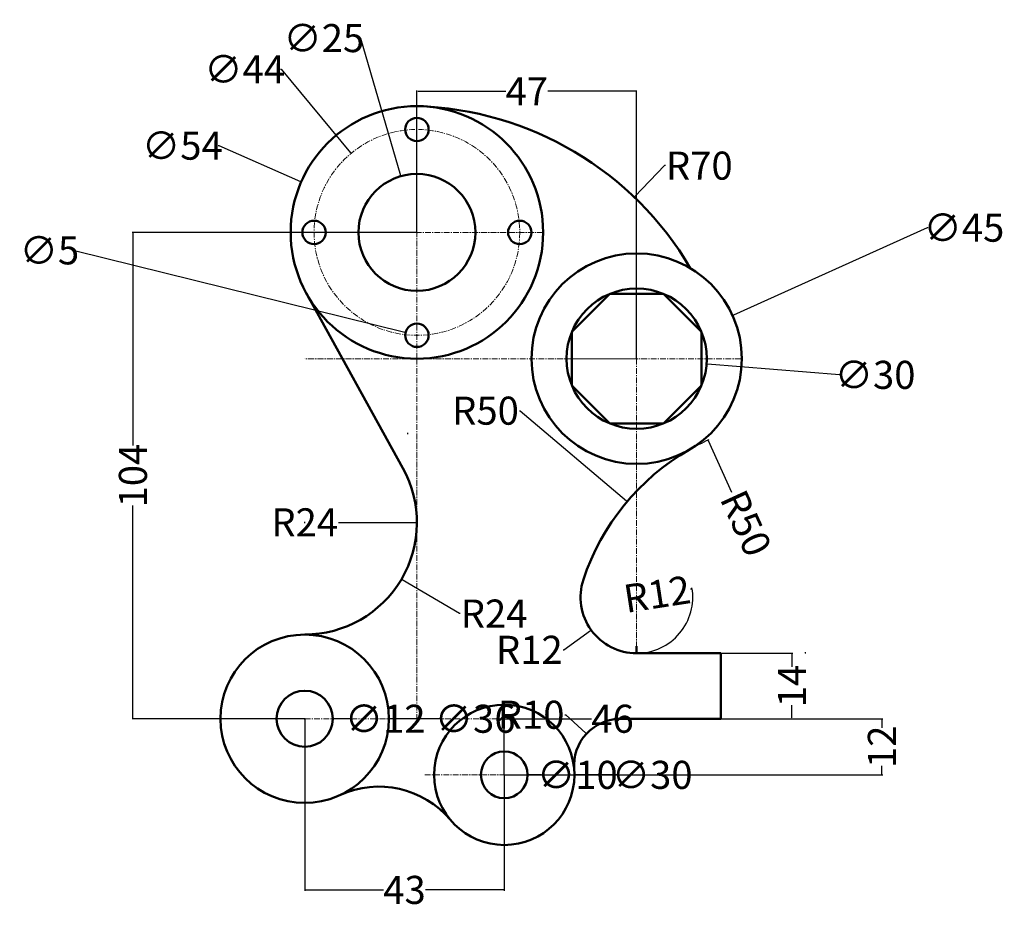
# Model space of a CAD drawing. Units: millimetres. Extents: x 65 to 276, y -19 to 171.
import ezdxf

# ---------------------------------------------------------------- set-up
doc = ezdxf.new("R2010")
doc.units = ezdxf.units.MM
doc.header["$MEASUREMENT"] = 0
doc.linetypes.add('CENTER', pattern=[2, 1.25, -0.25, 0.25, -0.25])
for name, color, linetype, lineweight in [('M-CNTR', 1, 'CENTER', 18), ('M-CONS', 8, 'Continuous', 13), ('M-DIMS', 2, 'Continuous', 25), ('M-OUTL', 7, 'Continuous', 50)]:
    doc.layers.add(name, color=color, linetype=linetype, lineweight=lineweight)
doc.styles.get("Standard").update_dxf_attribs({"font": 'arial.ttf'})
doc.dimstyles.get("Standard").update_dxf_attribs({"dimtxt": 6, "dimasz": 0.18, "dimexe": 0.18, "dimexo": 0.0625, "dimgap": 0.09, "dimtad": 0, "dimtoh": 1, "dimdec": 0, "dimzin": 0, "dimdsep": 46, "dimtxsty": 'Standard', "dimcen": 0.09, "dimadec": 0, "dimazin": 0, "dimtfac": 1, "dimtdec": 0, "dimtofl": 0, "dimtmove": 0, "dimatfit": 3, "dimfxl": 1, "dimtolj": 1, "dimtzin": 0, "dimarcsym": 0})

# ---------------------------------------------------------------- blocks, each defined once
blk = doc.blocks.new('*D1')
at = {"layer": 'Defpoints', "color": 0, "transparency": 16777216}
for p in [(196.83, 132.98), (148.37, 82.46)]:
    blk.add_point(p, dxfattribs=at)
at = {"layer": 'M-DIMS', "color": 0, "lineweight": -2, "transparency": 16777216}
for p, q in [((203.3, 139.72), (196.95, 133.11)), ((203.48, 139.72), (203.3, 139.72)), ((148.28, 82.46), (148.46, 82.46)), ((148.37, 82.37), (148.37, 82.55))]:
    blk.add_line(p, q, dxfattribs=at)
at = {"layer": 'M-DIMS', "color": 0, "transparency": 16777216}
blk.add_solid([(196.93, 133.13), (196.97, 133.09), (196.83, 132.98)], dxfattribs=at)
at = {"layer": 'M-DIMS', "color": 0, "transparency": 16777216, "insert": (210.73, 139.72), "char_height": 6, "attachment_point": 5}
blk.add_mtext('\\A1;R70', dxfattribs=at)
blk = doc.blocks.new('*D2')
at = {"layer": 'Defpoints', "color": 0, "transparency": 16777216}
for p in [(212.6, 81.02), (233.43, 35.56)]:
    blk.add_point(p, dxfattribs=at)
at = {"layer": 'M-DIMS', "color": 0, "lineweight": -2, "transparency": 16777216}
blk.add_line((217.71, 69.85), (212.67, 80.85), dxfattribs=at)
blk.add_arc((233.43, 35.56), 50, 114.4144, 119.7887, dxfattribs=at)
at = {"layer": 'M-DIMS', "color": 0, "transparency": 16777216}
blk.add_solid([(212.7, 80.86), (212.65, 80.84), (212.6, 81.02)], dxfattribs=at)
at = {"layer": 'M-DIMS', "color": 0, "transparency": 16777216, "insert": (220.73, 63.26), "char_height": 6, "attachment_point": 5, "rotation": 294.6207}
blk.add_mtext('\\A1;R50', dxfattribs=at)
blk = doc.blocks.new('*D3')
at = {"layer": 'Defpoints', "color": 0, "transparency": 16777216}
for p in [(209.19, 49.25), (197.33, 47.44)]:
    blk.add_point(p, dxfattribs=at)
at = {"layer": 'M-DIMS', "color": 0, "lineweight": -2, "transparency": 16777216}
blk.add_line((208.84, 49.2), (209.01, 49.23), dxfattribs=at)
blk.add_arc((197.33, 47.44), 12, 270.2984, 9.5776, dxfattribs=at)
at = {"layer": 'M-DIMS', "color": 0, "transparency": 16777216}
blk.add_solid([(209.01, 49.26), (209.02, 49.2), (209.19, 49.25)], dxfattribs=at)
at = {"layer": 'M-DIMS', "color": 0, "transparency": 16777216, "insert": (201.69, 48.1), "char_height": 6, "attachment_point": 5, "rotation": 8.7182}
blk.add_mtext('\\A1;R12', dxfattribs=at)
blk = doc.blocks.new('*D4')
at = {"layer": 'Defpoints', "color": 0, "transparency": 16777216}
for p in [(126.33, 63.44), (150.33, 63.44)]:
    blk.add_point(p, dxfattribs=at)
at = {"layer": 'M-DIMS', "color": 0, "lineweight": -2, "transparency": 16777216}
blk.add_line((133.58, 63.44), (150.15, 63.44), dxfattribs=at)
at = {"layer": 'M-DIMS', "color": 0, "transparency": 16777216}
blk.add_solid([(150.15, 63.47), (150.15, 63.41), (150.33, 63.44)], dxfattribs=at)
at = {"layer": 'M-DIMS', "color": 0, "transparency": 16777216, "insert": (126.33, 63.44), "char_height": 6, "attachment_point": 5}
blk.add_mtext('\\A1;R24', dxfattribs=at)
blk = doc.blocks.new('*D5')
at = {"layer": 'Defpoints', "color": 0, "transparency": 16777216}
for p in [(150.33, 125.44), (89.58, 21.44), (126.33, 21.44)]:
    blk.add_point(p, dxfattribs=at)
at = {"layer": 'M-DIMS', "color": 0, "lineweight": -2, "transparency": 16777216}
for p, q in [((150.27, 125.44), (89.4, 125.44)), ((89.58, 125.26), (89.58, 79.86)), ((89.58, 21.62), (89.58, 67.01)), ((126.27, 21.44), (89.4, 21.44))]:
    blk.add_line(p, q, dxfattribs=at)
at = {"layer": 'M-DIMS', "color": 0, "transparency": 16777216}
for points in [[(89.55, 125.26), (89.61, 125.26), (89.58, 125.44)], [(89.55, 21.62), (89.61, 21.62), (89.58, 21.44)]]:
    blk.add_solid(points, dxfattribs=at)
at = {"layer": 'M-DIMS', "color": 0, "transparency": 16777216, "insert": (89.58, 73.44), "char_height": 6, "attachment_point": 5, "rotation": 90}
blk.add_mtext('\\A1;104', dxfattribs=at)
blk = doc.blocks.new('*D6')
at = {"layer": 'Defpoints', "color": 0, "transparency": 16777216}
for p in [(197.33, 155.62), (150.33, 125.44), (197.33, 98.44)]:
    blk.add_point(p, dxfattribs=at)
at = {"layer": 'M-DIMS', "color": 0, "lineweight": -2, "transparency": 16777216}
for p, q in [((150.33, 125.5), (150.33, 155.8)), ((150.51, 155.62), (169.32, 155.62)), ((197.15, 155.62), (178.34, 155.62)), ((197.33, 98.5), (197.33, 155.8))]:
    blk.add_line(p, q, dxfattribs=at)
at = {"layer": 'M-DIMS', "color": 0, "transparency": 16777216}
for points in [[(150.51, 155.65), (150.51, 155.59), (150.33, 155.62)], [(197.15, 155.65), (197.15, 155.59), (197.33, 155.62)]]:
    blk.add_solid(points, dxfattribs=at)
at = {"layer": 'M-DIMS', "color": 0, "transparency": 16777216, "insert": (173.83, 155.62), "char_height": 6, "attachment_point": 5}
blk.add_mtext('\\A1;47', dxfattribs=at)
blk = doc.blocks.new('*D7')
at = {"layer": 'Defpoints', "color": 0, "transparency": 16777216}
for p in [(126.33, 21.44), (169.01, 9.44), (169.01, -15.16)]:
    blk.add_point(p, dxfattribs=at)
at = {"layer": 'M-DIMS', "color": 0, "lineweight": -2, "transparency": 16777216}
for p, q in [((126.33, 21.37), (126.33, -15.34)), ((169.01, 9.37), (169.01, -15.34)), ((126.51, -15.16), (143.16, -15.16)), ((168.83, -15.16), (152.18, -15.16))]:
    blk.add_line(p, q, dxfattribs=at)
at = {"layer": 'M-DIMS', "color": 0, "transparency": 16777216}
for points in [[(126.51, -15.13), (126.51, -15.19), (126.33, -15.16)], [(168.83, -15.13), (168.83, -15.19), (169.01, -15.16)]]:
    blk.add_solid(points, dxfattribs=at)
at = {"layer": 'M-DIMS', "color": 0, "transparency": 16777216, "insert": (147.67, -15.16), "char_height": 6, "attachment_point": 5}
blk.add_mtext('\\A1;43', dxfattribs=at)
blk = doc.blocks.new('*D8')
at = {"layer": 'Defpoints', "color": 0, "transparency": 16777216}
for p in [(215.33, 21.44), (215.33, 21.44), (169.01, 9.44)]:
    blk.add_point(p, dxfattribs=at)
at = {"layer": 'M-DIMS', "color": 0, "lineweight": -2, "transparency": 16777216}
for p, q in [((169.01, 9.5), (169.01, 21.62)), ((169.19, 21.44), (187.67, 21.44)), ((215.15, 21.44), (196.68, 21.44)), ((215.33, 21.5), (215.33, 21.62))]:
    blk.add_line(p, q, dxfattribs=at)
at = {"layer": 'M-DIMS', "color": 0, "transparency": 16777216}
for points in [[(169.19, 21.47), (169.19, 21.41), (169.01, 21.44)], [(215.15, 21.47), (215.15, 21.41), (215.33, 21.44)]]:
    blk.add_solid(points, dxfattribs=at)
at = {"layer": 'M-DIMS', "color": 0, "transparency": 16777216, "insert": (192.17, 21.44), "char_height": 6, "attachment_point": 5}
blk.add_mtext('\\A1;46', dxfattribs=at)
blk = doc.blocks.new('*D9')
at = {"layer": 'Defpoints', "color": 0, "transparency": 16777216}
for p in [(215.33, 21.44), (249.78, 21.44), (169.01, 9.44)]:
    blk.add_point(p, dxfattribs=at)
at = {"layer": 'M-DIMS', "color": 0, "lineweight": -2, "transparency": 16777216}
for p, q in [((215.39, 21.44), (249.96, 21.44)), ((249.78, 21.26), (249.78, 19.51)), ((249.78, 9.62), (249.78, 11.36)), ((169.07, 9.44), (249.96, 9.44))]:
    blk.add_line(p, q, dxfattribs=at)
at = {"layer": 'M-DIMS', "color": 0, "transparency": 16777216}
for points in [[(249.75, 21.26), (249.81, 21.26), (249.78, 21.44)], [(249.75, 9.62), (249.81, 9.62), (249.78, 9.44)]]:
    blk.add_solid(points, dxfattribs=at)
at = {"layer": 'M-DIMS', "color": 0, "transparency": 16777216, "insert": (249.78, 15.44), "char_height": 6, "attachment_point": 5, "rotation": 90}
blk.add_mtext('\\A1;12', dxfattribs=at)
blk = doc.blocks.new('*D10')
at = {"layer": 'Defpoints', "color": 0, "transparency": 16777216}
for p in [(125.6, 136.27), (175.06, 114.6)]:
    blk.add_point(p, dxfattribs=at)
at = {"layer": 'M-DIMS', "color": 0, "lineweight": -2, "transparency": 16777216}
for p, q in [((107.8, 143.99), (107.98, 143.99)), ((107.98, 143.99), (125.44, 136.35)), ((150.24, 125.44), (150.42, 125.44)), ((150.33, 125.35), (150.33, 125.53))]:
    blk.add_line(p, q, dxfattribs=at)
at = {"layer": 'M-DIMS', "color": 0, "transparency": 16777216}
blk.add_solid([(125.45, 136.37), (125.42, 136.32), (125.6, 136.27)], dxfattribs=at)
at = {"layer": 'M-DIMS', "color": 0, "transparency": 16777216, "insert": (100.16, 143.99), "char_height": 6, "attachment_point": 5}
blk.add_mtext('\\A1;∅54', dxfattribs=at)
blk = doc.blocks.new('*D11')
at = {"layer": 'Defpoints', "color": 0, "transparency": 16777216}
for p in [(136.27, 142.35), (164.4, 108.52)]:
    blk.add_point(p, dxfattribs=at)
at = {"layer": 'M-DIMS', "color": 0, "lineweight": -2, "transparency": 16777216}
for p, q in [((121.13, 160.33), (121.31, 160.33)), ((121.31, 160.33), (136.15, 142.49)), ((150.24, 125.44), (150.42, 125.44)), ((150.33, 125.35), (150.33, 125.53))]:
    blk.add_line(p, q, dxfattribs=at)
at = {"layer": 'M-DIMS', "color": 0, "transparency": 16777216}
blk.add_solid([(136.17, 142.51), (136.13, 142.47), (136.27, 142.35)], dxfattribs=at)
at = {"layer": 'M-DIMS', "color": 0, "transparency": 16777216, "insert": (113.49, 160.33), "char_height": 6, "attachment_point": 5}
blk.add_mtext('\\A1;∅44', dxfattribs=at)
blk = doc.blocks.new('*D12')
at = {"layer": 'Defpoints', "color": 0, "transparency": 16777216}
for p in [(146.85, 137.44), (153.81, 113.43)]:
    blk.add_point(p, dxfattribs=at)
at = {"layer": 'M-DIMS', "color": 0, "lineweight": -2, "transparency": 16777216}
for p, q in [((138.1, 166.99), (138.28, 166.99)), ((138.28, 166.99), (146.8, 137.61)), ((150.24, 125.44), (150.42, 125.44)), ((150.33, 125.35), (150.33, 125.53))]:
    blk.add_line(p, q, dxfattribs=at)
at = {"layer": 'M-DIMS', "color": 0, "transparency": 16777216}
blk.add_solid([(146.83, 137.62), (146.77, 137.61), (146.85, 137.44)], dxfattribs=at)
at = {"layer": 'M-DIMS', "color": 0, "transparency": 16777216, "insert": (130.43, 166.99), "char_height": 6, "attachment_point": 5}
blk.add_mtext('\\A1;∅25', dxfattribs=at)
blk = doc.blocks.new('*D13')
at = {"layer": 'Defpoints', "color": 0, "transparency": 16777216}
for p in [(147.9, 104.04), (152.76, 102.83)]:
    blk.add_point(p, dxfattribs=at)
at = {"layer": 'M-DIMS', "color": 0, "lineweight": -2, "transparency": 16777216}
for p, q in [((77.08, 121.6), (147.73, 104.08)), ((150.24, 103.44), (150.42, 103.44)), ((150.33, 103.35), (150.33, 103.53))]:
    blk.add_line(p, q, dxfattribs=at)
at = {"layer": 'M-DIMS', "color": 0, "transparency": 16777216}
blk.add_solid([(147.74, 104.11), (147.72, 104.05), (147.9, 104.04)], dxfattribs=at)
at = {"layer": 'M-DIMS', "color": 0, "transparency": 16777216, "insert": (71.73, 121.6), "char_height": 6, "attachment_point": 5}
blk.add_mtext('\\A1;∅5', dxfattribs=at)
blk = doc.blocks.new('*D14')
at = {"layer": 'Defpoints', "color": 0, "transparency": 16777216}
for p in [(217.84, 107.68), (176.82, 89.19)]:
    blk.add_point(p, dxfattribs=at)
at = {"layer": 'M-DIMS', "color": 0, "lineweight": -2, "transparency": 16777216}
for p, q in [((259.48, 126.45), (218.01, 107.76)), ((259.66, 126.45), (259.48, 126.45)), ((197.24, 98.44), (197.42, 98.44)), ((197.33, 98.35), (197.33, 98.53))]:
    blk.add_line(p, q, dxfattribs=at)
at = {"layer": 'M-DIMS', "color": 0, "transparency": 16777216}
blk.add_solid([(218, 107.78), (218.02, 107.73), (217.84, 107.68)], dxfattribs=at)
at = {"layer": 'M-DIMS', "color": 0, "transparency": 16777216, "insert": (267.33, 126.45), "char_height": 6, "attachment_point": 5}
blk.add_mtext('\\A1;∅45', dxfattribs=at)
blk = doc.blocks.new('*D15')
at = {"layer": 'Defpoints', "color": 0, "transparency": 16777216}
for p in [(182.38, 99.63), (212.28, 97.24)]:
    blk.add_point(p, dxfattribs=at)
at = {"layer": 'M-DIMS', "color": 0, "lineweight": -2, "transparency": 16777216}
for p, q in [((197.24, 98.44), (197.42, 98.44)), ((197.33, 98.35), (197.33, 98.53)), ((240.69, 94.98), (212.46, 97.23))]:
    blk.add_line(p, q, dxfattribs=at)
at = {"layer": 'M-DIMS', "color": 0, "transparency": 16777216}
blk.add_solid([(212.47, 97.26), (212.46, 97.2), (212.28, 97.24)], dxfattribs=at)
at = {"layer": 'M-DIMS', "color": 0, "transparency": 16777216, "insert": (248.33, 94.98), "char_height": 6, "attachment_point": 5}
blk.add_mtext('\\A1;∅30', dxfattribs=at)
blk = doc.blocks.new('*D16')
at = {"layer": 'Defpoints', "color": 0, "transparency": 16777216}
for p in [(215.33, 35.44), (215.33, 21.44), (230.53, 21.44)]:
    blk.add_point(p, dxfattribs=at)
at = {"layer": 'M-DIMS', "color": 0, "lineweight": -2, "transparency": 16777216}
for p, q in [((215.39, 35.44), (230.71, 35.44)), ((230.53, 35.26), (230.53, 32.53)), ((230.53, 21.62), (230.53, 24.34)), ((215.39, 21.44), (230.71, 21.44))]:
    blk.add_line(p, q, dxfattribs=at)
at = {"layer": 'M-DIMS', "color": 0, "transparency": 16777216}
for points in [[(230.5, 35.26), (230.56, 35.26), (230.53, 35.44)], [(230.5, 21.62), (230.56, 21.62), (230.53, 21.44)]]:
    blk.add_solid(points, dxfattribs=at)
at = {"layer": 'M-DIMS', "color": 0, "transparency": 16777216, "insert": (230.53, 28.44), "char_height": 6, "attachment_point": 5, "rotation": 90}
blk.add_mtext('\\A1;14', dxfattribs=at)
blk = doc.blocks.new('*D17')
at = {"layer": 'Defpoints', "color": 0, "transparency": 16777216}
for p in [(154.01, 9.44), (184.01, 9.44)]:
    blk.add_point(p, dxfattribs=at)
at = {"layer": 'M-DIMS', "color": 0, "lineweight": -2, "transparency": 16777216}
for p, q in [((168.92, 9.44), (169.1, 9.44)), ((169.01, 9.35), (169.01, 9.53)), ((193.01, 9.44), (184.19, 9.44))]:
    blk.add_line(p, q, dxfattribs=at)
at = {"layer": 'M-DIMS', "color": 0, "transparency": 16777216}
blk.add_solid([(184.19, 9.47), (184.19, 9.41), (184.01, 9.44)], dxfattribs=at)
at = {"layer": 'M-DIMS', "color": 0, "transparency": 16777216, "insert": (200.65, 9.44), "char_height": 6, "attachment_point": 5}
blk.add_mtext('\\A1;∅30', dxfattribs=at)
blk = doc.blocks.new('*D18')
at = {"layer": 'Defpoints', "color": 0, "transparency": 16777216}
for p in [(108.33, 21.44), (144.33, 21.44)]:
    blk.add_point(p, dxfattribs=at)
at = {"layer": 'M-DIMS', "color": 0, "lineweight": -2, "transparency": 16777216}
for p, q in [((126.24, 21.44), (126.42, 21.44)), ((126.33, 21.35), (126.33, 21.53)), ((155.13, 21.44), (144.51, 21.44))]:
    blk.add_line(p, q, dxfattribs=at)
at = {"layer": 'M-DIMS', "color": 0, "transparency": 16777216}
blk.add_solid([(144.51, 21.47), (144.51, 21.41), (144.33, 21.44)], dxfattribs=at)
at = {"layer": 'M-DIMS', "color": 0, "transparency": 16777216, "insert": (162.78, 21.44), "char_height": 6, "attachment_point": 5}
blk.add_mtext('\\A1;∅36', dxfattribs=at)
blk = doc.blocks.new('*D19')
at = {"layer": 'Defpoints', "color": 0, "transparency": 16777216}
for p in [(120.33, 21.44), (132.33, 21.44)]:
    blk.add_point(p, dxfattribs=at)
at = {"layer": 'M-DIMS', "color": 0, "lineweight": -2, "transparency": 16777216}
for p, q in [((126.24, 21.44), (126.42, 21.44)), ((126.33, 21.35), (126.33, 21.53)), ((135.93, 21.44), (132.51, 21.44))]:
    blk.add_line(p, q, dxfattribs=at)
at = {"layer": 'M-DIMS', "color": 0, "transparency": 16777216}
blk.add_solid([(132.51, 21.47), (132.51, 21.41), (132.33, 21.44)], dxfattribs=at)
at = {"layer": 'M-DIMS', "color": 0, "transparency": 16777216, "insert": (143.55, 21.44), "char_height": 6, "attachment_point": 5}
blk.add_mtext('\\A1;∅12', dxfattribs=at)
blk = doc.blocks.new('*D20')
at = {"layer": 'Defpoints', "color": 0, "transparency": 16777216}
for p in [(164.01, 9.44), (174.01, 9.44)]:
    blk.add_point(p, dxfattribs=at)
at = {"layer": 'M-DIMS', "color": 0, "lineweight": -2, "transparency": 16777216}
for p, q in [((168.92, 9.44), (169.1, 9.44)), ((169.01, 9.35), (169.01, 9.53)), ((177.01, 9.44), (174.19, 9.44))]:
    blk.add_line(p, q, dxfattribs=at)
at = {"layer": 'M-DIMS', "color": 0, "transparency": 16777216}
blk.add_solid([(174.19, 9.47), (174.19, 9.41), (174.01, 9.44)], dxfattribs=at)
at = {"layer": 'M-DIMS', "color": 0, "transparency": 16777216, "insert": (184.65, 9.44), "char_height": 6, "attachment_point": 5}
blk.add_mtext('\\A1;∅10', dxfattribs=at)
blk = doc.blocks.new('*D21')
at = {"layer": 'Defpoints', "color": 0, "transparency": 16777216}
for p in [(126.33, 63.44), (147, 51.24)]:
    blk.add_point(p, dxfattribs=at)
at = {"layer": 'M-DIMS', "color": 0, "lineweight": -2, "transparency": 16777216}
for p, q in [((126.24, 63.44), (126.42, 63.44)), ((126.33, 63.35), (126.33, 63.53)), ((159.41, 43.93), (147.16, 51.15)), ((159.59, 43.93), (159.41, 43.93))]:
    blk.add_line(p, q, dxfattribs=at)
at = {"layer": 'M-DIMS', "color": 0, "transparency": 16777216}
blk.add_solid([(147.17, 51.18), (147.14, 51.13), (147, 51.24)], dxfattribs=at)
at = {"layer": 'M-DIMS', "color": 0, "transparency": 16777216, "insert": (166.83, 43.93), "char_height": 6, "attachment_point": 5}
blk.add_mtext('\\A1;R24', dxfattribs=at)
blk = doc.blocks.new('*D22')
at = {"layer": 'Defpoints', "color": 0, "transparency": 16777216}
for p in [(197.33, 47.44), (187.61, 40.4)]:
    blk.add_point(p, dxfattribs=at)
at = {"layer": 'M-DIMS', "color": 0, "lineweight": -2, "transparency": 16777216}
for p, q in [((197.24, 47.44), (197.42, 47.44)), ((197.33, 47.35), (197.33, 47.53)), ((181.78, 36.18), (187.46, 40.29)), ((181.6, 36.18), (181.78, 36.18))]:
    blk.add_line(p, q, dxfattribs=at)
at = {"layer": 'M-DIMS', "color": 0, "transparency": 16777216}
blk.add_solid([(187.45, 40.32), (187.48, 40.27), (187.61, 40.4)], dxfattribs=at)
at = {"layer": 'M-DIMS', "color": 0, "transparency": 16777216, "insert": (174.37, 36.18), "char_height": 6, "attachment_point": 5}
blk.add_mtext('\\A1;R12', dxfattribs=at)
blk = doc.blocks.new('*D23')
at = {"layer": 'Defpoints', "color": 0, "transparency": 16777216}
for p in [(186.58, 18.22), (193.93, 11.44)]:
    blk.add_point(p, dxfattribs=at)
at = {"layer": 'M-DIMS', "color": 0, "lineweight": -2, "transparency": 16777216}
for p, q in [((181.99, 22.29), (182.17, 22.29)), ((182.17, 22.29), (186.45, 18.34)), ((193.84, 11.44), (194.02, 11.44)), ((193.93, 11.35), (193.93, 11.53))]:
    blk.add_line(p, q, dxfattribs=at)
at = {"layer": 'M-DIMS', "color": 0, "transparency": 16777216}
blk.add_solid([(186.47, 18.36), (186.43, 18.32), (186.58, 18.22)], dxfattribs=at)
at = {"layer": 'M-DIMS', "color": 0, "transparency": 16777216, "insert": (174.75, 22.29), "char_height": 6, "attachment_point": 5}
blk.add_mtext('\\A1;R10', dxfattribs=at)
blk = doc.blocks.new('*D24')
at = {"layer": 'Defpoints', "color": 0, "transparency": 16777216}
for p in [(195.3, 67.91), (233.43, 35.56)]:
    blk.add_point(p, dxfattribs=at)
at = {"layer": 'M-DIMS', "color": 0, "lineweight": -2, "transparency": 16777216}
for p, q in [((172.25, 87.32), (172.43, 87.32)), ((172.43, 87.32), (195.17, 68.03)), ((233.34, 35.56), (233.52, 35.56)), ((233.43, 35.47), (233.43, 35.65))]:
    blk.add_line(p, q, dxfattribs=at)
at = {"layer": 'M-DIMS', "color": 0, "transparency": 16777216}
blk.add_solid([(195.18, 68.05), (195.15, 68), (195.3, 67.91)], dxfattribs=at)
at = {"layer": 'M-DIMS', "color": 0, "transparency": 16777216, "insert": (165, 87.32), "char_height": 6, "attachment_point": 5}
blk.add_mtext('\\A1;R50', dxfattribs=at)

msp = doc.modelspace()

# ---------------------------------------------------------------- linework, layer by layer
at = {"layer": 'M-CNTR'}
for p, q in [((150.33, 98.44), (150.33, 152.44)), ((177.33, 125.44), (123.33, 125.44)), ((197.33, 98.44), (197.33, 120.94)), ((150.33, 98.44), (126.33, 98.44)), ((150.33, 98.44), (219.83, 98.44)), ((150.33, 98.44), (150.33, 21.44)), ((197.33, 98.44), (182.33, 98.44)), ((197.33, 98.44), (197.33, 75.94)), ((197.33, 98.44), (197.33, 75.94)), ((197.33, 75.94), (197.33, 36.94)), ((126.33, 21.44), (178.01, 21.44)), ((152.01, 9.44), (169.01, 9.44))]:
    msp.add_line(p, q, dxfattribs=at)
msp.add_circle((150.33, 125.44), 22, dxfattribs=at)
at = {"layer": 'M-CONS'}
msp.add_lwpolyline([(197.33, 98.44), (197.33, 98.44), (197.33, 98.44), (197.33, 98.44), (197.33, 98.44), (197.33, 98.44), (197.33, 98.44), (197.33, 98.44)], close=True, dxfattribs=at)
at = {"layer": 'M-OUTL'}
for p, q in [((126.7, 112.37), (147.34, 75.05)), ((197.33, 35.44), (197.33, 36.94)), ((215.33, 35.44), (197.33, 35.44)), ((215.33, 21.44), (215.33, 35.44)), ((193.93, 21.44), (215.33, 21.44))]:
    msp.add_line(p, q, dxfattribs=at)
msp.add_lwpolyline([(191.59, 112.29), (183.47, 104.18), (183.47, 92.7), (191.59, 84.58), (203.07, 84.58), (211.19, 92.7), (211.19, 104.18), (203.07, 112.29)], close=True, dxfattribs=at)
for centre, radius in [((150.33, 125.44), 27), ((150.33, 147.44), 2.5), ((150.33, 125.44), 12.5), ((128.33, 125.44), 2.5), ((172.33, 125.44), 2.5), ((197.33, 98.44), 22.5), ((197.33, 98.44), 15), ((150.33, 103.44), 2.5), ((126.33, 21.44), 18), ((126.33, 21.44), 6), ((169.01, 9.44), 15), ((169.01, 9.44), 5)]:
    msp.add_circle(centre, radius, dxfattribs=at)
for centre, radius, start, end in [((148.37, 82.46), 70, 30.3123, 88.3947), ((233.43, 35.56), 50, 119.8604, 161.79), ((126.33, 63.44), 24, 270, 28.934), ((197.33, 47.44), 12, 161.79, 270), ((193.93, 11.44), 10, 90, 184.5886), ((142.22, -13.08), 20, 40.0467, 114.714)]:
    msp.add_arc(centre, radius, start, end, dxfattribs=at)

# ---------------------------------------------------------------- dimensions: what is measured, and where the dimension line sits
at = {"layer": 'M-DIMS'}
for p1, p2, override, picture, middle in [((153.81, 113.43), (146.85, 137.44), {"dimclrd": 0, "dimclre": 0, "dimclrt": 0}, '*D12', (130.43, 166.99)), ((164.4, 108.52), (136.27, 142.35), {"dimclrd": 0, "dimclre": 0, "dimclrt": 0}, '*D11', (113.49, 160.33)), ((175.06, 114.6), (125.6, 136.27), {"dimclrd": 0, "dimclre": 0, "dimclrt": 0}, '*D10', (100.16, 143.99)), ((176.82, 89.19), (217.84, 107.68), {"dimclrd": 0, "dimclre": 0, "dimclrt": 0}, '*D14', (267.33, 126.45)), ((152.76, 102.83), (147.9, 104.04), {"dimclrd": 0, "dimclre": 0, "dimclrt": 0}, '*D13', (77.08, 121.6)), ((182.38, 99.63), (212.28, 97.24), {"dimclrd": 0, "dimclre": 0, "dimclrt": 0}, '*D15', (240.69, 94.98)), ((108.33, 21.44), (144.33, 21.44), {"dimdec": 0, "dimlfac": 1, "dimrnd": 0, "dimzin": 0, "dimdsep": 46, "dimlunit": 2}, '*D18', (155.13, 21.44)), ((120.33, 21.44), (132.33, 21.44), {"dimdec": 0, "dimlfac": 1, "dimrnd": 0, "dimzin": 0, "dimdsep": 46, "dimlunit": 2}, '*D19', (135.93, 21.44)), ((154.01, 9.44), (184.01, 9.44), {"dimdec": 0, "dimlfac": 1, "dimrnd": 0, "dimzin": 0, "dimdsep": 46, "dimlunit": 2}, '*D17', (193.01, 9.44)), ((164.01, 9.44), (174.01, 9.44), {"dimdec": 0, "dimlfac": 1, "dimrnd": 0, "dimzin": 0, "dimdsep": 46, "dimlunit": 2}, '*D20', (177.01, 9.44))]:
    dim = msp.add_diameter_dim_2p(p1=p1, p2=p2, dimstyle='Standard', override=override, dxfattribs=at)
    dim.commit()
    dim.dimension.update_dxf_attribs({"geometry": picture, "text_midpoint": middle, "dimtype": 163})
for base, p1, p2, picture, middle in [((197.33, 155.62), (150.33, 125.44), (197.33, 98.44), '*D6', (173.83, 155.62)), ((215.33, 21.44), (169.01, 9.44), (215.33, 21.44), '*D8', (192.17, 21.44)), ((169.01, -15.16), (126.33, 21.44), (169.01, 9.44), '*D7', (147.67, -15.16))]:
    dim = msp.add_linear_dim(base=base, p1=p1, p2=p2, dimstyle='Standard', override={"dimclrd": 0, "dimclre": 0, "dimclrt": 0}, dxfattribs=at)
    dim.commit()
    dim.dimension.update_dxf_attribs({"geometry": picture, "text_midpoint": middle})
for center, mpoint, override, picture, middle in [((148.37, 82.46), (196.83, 132.98), {"dimclrd": 0, "dimclre": 0, "dimclrt": 0}, '*D1', (210.73, 139.72)), ((233.43, 35.56), (195.3, 67.91), {"dimdec": 0, "dimlfac": 1, "dimrnd": 0, "dimzin": 0, "dimdsep": 46, "dimlunit": 2}, '*D24', (165, 87.32)), ((233.43, 35.56), (212.6, 81.02), {"dimclrd": 0, "dimclre": 0, "dimclrt": 0}, '*D2', (220.73, 63.26)), ((126.33, 63.44), (150.33, 63.44), {"dimclrd": 0, "dimclre": 0, "dimclrt": 0}, '*D4', (126.33, 63.44)), ((126.33, 63.44), (147, 51.24), {"dimdec": 0, "dimlfac": 1, "dimrnd": 0, "dimzin": 0, "dimdsep": 46, "dimlunit": 2}, '*D21', (166.83, 43.93)), ((197.33, 47.44), (209.19, 49.25), {"dimclrd": 0, "dimclre": 0, "dimclrt": 0}, '*D3', (201.69, 48.1)), ((197.33, 47.44), (187.61, 40.4), {"dimdec": 0, "dimlfac": 1, "dimrnd": 0, "dimzin": 0, "dimdsep": 46, "dimlunit": 2}, '*D22', (174.37, 36.18)), ((193.93, 11.44), (186.58, 18.22), {"dimdec": 0, "dimlfac": 1, "dimrnd": 0, "dimzin": 0, "dimdsep": 46, "dimlunit": 2}, '*D23', (174.75, 22.29))]:
    dim = msp.add_radius_dim(center=center, mpoint=mpoint, dimstyle='Standard', override=override, dxfattribs=at)
    dim.commit()
    dim.dimension.update_dxf_attribs({"geometry": picture, "text_midpoint": middle, "dimtype": 164})
for base, p1, p2, override, picture, middle in [((89.58, 21.44), (150.33, 125.44), (126.33, 21.44), {"dimclrd": 0, "dimclre": 0, "dimclrt": 0}, '*D5', (89.58, 73.44)), ((230.53, 21.44), (215.33, 35.44), (215.33, 21.44), {"dimdec": 0, "dimlfac": 1, "dimrnd": 0, "dimzin": 0, "dimdsep": 46, "dimlunit": 2}, '*D16', (230.53, 28.44)), ((249.78, 21.44), (169.01, 9.44), (215.33, 21.44), {"dimclrd": 0, "dimclre": 0, "dimclrt": 0}, '*D9', (249.78, 15.44))]:
    dim = msp.add_linear_dim(base=base, p1=p1, p2=p2, angle=90, dimstyle='Standard', override=override, dxfattribs=at)
    dim.commit()
    dim.dimension.update_dxf_attribs({"geometry": picture, "text_midpoint": middle})

doc.saveas('drawing.dxf')
